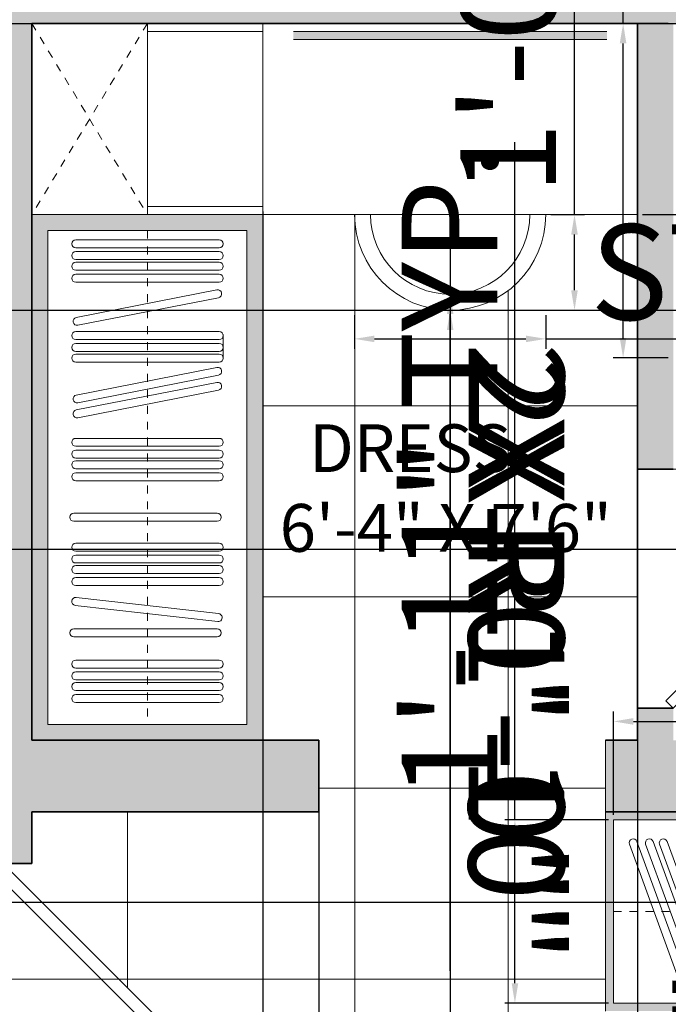
# Model space of a CAD drawing. Units: millimetres. Extents: x 542930 to 543750, y 628093 to 628738.
# Tile 9 of 14: x 543333 to 543414, y 628458 to 628581. Entities that reach past the tile are written whole.
import ezdxf

# ---------------------------------------------------------------- set-up
doc = ezdxf.new("R2010")
doc.units = ezdxf.units.MM
doc.linetypes.add('JIS_02_1.0', pattern=[2, 1, -1])
for name, color, linetype, lineweight in [('A-ANNO-DIMS', 2, 'Continuous', 18), ('A-FURN', 8, 'Continuous', 18), ('A-FURN-MILL', 8, 'Continuous', 18), ('A-FURN-MILL-HIDN', 8, 'JIS_02_1.0', 13), ('A-FURN-PATT', 9, 'Continuous', 13), ('A-WALL', 7, 'Continuous', 35), ('DOORS', 30, 'Continuous', 18)]:
    doc.layers.add(name, color=color, linetype=linetype, lineweight=lineweight)
for name, color, linetype, lineweight, true_color in [('A-AREA-IDEN', 40, 'Continuous', 18, 0xf8d731), ('A-FLOR-PATT', 241, 'Continuous', 13, 0xf7abae), ('A-WALL-PATT', 251, 'Continuous', 13, 0x636466)]:
    doc.layers.add(name, color=color, linetype=linetype, lineweight=lineweight, true_color=true_color)
doc.styles.get("Standard").update_dxf_attribs({"font": 'arial.ttf'})
doc.dimstyles.new('ISO-25', dxfattribs={"dimtxt": 12, "dimasz": 2.5, "dimexe": 1.25, "dimexo": 0.625, "dimtad": 1, "dimdec": 0, "dimlunit": 3, "dimtxsty": 'Standard', "dimcen": 2.5, "dimadec": 0, "dimazin": 0, "dimtfac": 1, "dimtdec": 0, "dimtmove": 0, "dimatfit": 3, "dimfxl": 1, "dimarcsym": 0})

# ---------------------------------------------------------------- blocks, each defined once
blk = doc.blocks.new('*U2')
for p, q in [((0, 0), (0, -6)), ((40, 0), (40, -6))]:
    blk.add_line(p, q)
blk.add_lwpolyline([(0, 0), (28.28, 28.28), (29.52, 27.05), (1.24, -1.24)], close=True)
blk.add_arc((0, 0), 40, 0, 45)
blk = doc.blocks.new('*U3')
for p, q in [((-40, 0), (-40, -6)), ((0, 0), (0, -6))]:
    blk.add_line(p, q)
blk.add_lwpolyline([(0, 0), (-28.28, 28.28), (-29.52, 27.05), (-1.24, -1.24)], close=True)
blk.add_arc((0, 0), 40, 135, 180)
blk = doc.blocks.new('WARDROBE-DRESS-RAIL')
for p, q in [((0, 0), (0, 62)), ((0, 62), (25, 62)), ((25, 0), (25, 62)), ((3.52, 60.83), (21.52, 60.83)), ((3.52, 59.83), (21.52, 59.83)), ((3.52, 59.35), (21.52, 59.35)), ((3.52, 58.35), (21.52, 58.35)), ((3.52, 58.02), (21.52, 58.02)), ((3.52, 57.02), (21.52, 57.02)), ((3.52, 56.51), (21.52, 56.51)), ((3.52, 55.51), (21.52, 55.51)), ((3.57, 51.08), (21.23, 54.55)), ((3.76, 50.1), (21.43, 53.57)), ((3.52, 49.31), (21.52, 49.31)), ((3.52, 48.31), (21.52, 48.31)), ((3.52, 47.82), (21.52, 47.82)), ((3.52, 46.82), (21.52, 46.82)), ((3.52, 46.49), (21.52, 46.49)), ((3.52, 45.49), (21.52, 45.49)), ((3.57, 41.35), (21.23, 44.82)), ((3.76, 40.37), (21.43, 43.84)), ((3.57, 39.47), (21.23, 42.94)), ((3.76, 38.49), (21.43, 41.96)), ((3.52, 35.91), (21.52, 35.91)), ((3.52, 34.91), (21.52, 34.91)), ((3.52, 34.43), (21.52, 34.43)), ((3.52, 33.43), (21.52, 33.43)), ((3.52, 33.1), (21.52, 33.1)), ((3.52, 32.1), (21.52, 32.1)), ((3.52, 31.59), (21.52, 31.59)), ((3.52, 30.59), (21.52, 30.59)), ((3.27, 26.51), (21.27, 26.51)), ((3.27, 25.51), (21.27, 25.51)), ((3.52, 22.74), (21.52, 22.74)), ((3.52, 21.74), (21.52, 21.74)), ((3.52, 21.26), (21.52, 21.26)), ((3.52, 20.26), (21.52, 20.26)), ((3.52, 19.93), (21.52, 19.93)), ((3.52, 18.93), (21.52, 18.93)), ((3.52, 18.42), (21.52, 18.42)), ((3.52, 17.42), (21.52, 17.42)), ((3.44, 14.93), (21.33, 12.92)), ((3.56, 15.93), (21.44, 13.91)), ((3.27, 11.99), (21.27, 11.99)), ((3.27, 10.99), (21.27, 10.99)), ((3.52, 8.06), (21.52, 8.06)), ((3.52, 7.06), (21.52, 7.06)), ((3.52, 6.58), (21.52, 6.58)), ((3.52, 5.58), (21.52, 5.58)), ((3.52, 5.25), (21.52, 5.25)), ((3.52, 4.25), (21.52, 4.25)), ((3.52, 3.74), (21.52, 3.74)), ((3.52, 2.74), (21.52, 2.74)), ((0, 0), (25, 0))]:
    blk.add_line(p, q)
for centre, start, end in [((3.52, 60.33), 90, 270), ((21.52, 60.33), 270, 90), ((3.52, 58.85), 90, 270), ((21.52, 58.85), 270, 90), ((3.52, 57.52), 90, 270), ((21.52, 57.52), 270, 90), ((3.52, 56.01), 90, 270), ((21.52, 56.01), 270, 90), ((21.33, 54.06), 281.1082, 101.1082), ((3.67, 50.59), 101.1082, 281.1082), ((3.52, 48.81), 90, 270), ((21.52, 48.81), 270, 90), ((3.52, 47.32), 90, 270), ((21.52, 47.32), 270, 90), ((3.52, 45.99), 90, 270), ((21.52, 45.99), 270, 90), ((21.33, 44.33), 281.1082, 101.1082), ((21.33, 42.45), 281.1082, 101.1082), ((3.67, 40.86), 101.1082, 281.1082), ((3.67, 38.98), 101.1082, 281.1082), ((3.52, 35.41), 90, 270), ((21.52, 35.41), 270, 90), ((3.52, 33.93), 90, 270), ((21.52, 33.93), 270, 90), ((3.52, 32.6), 90, 270), ((21.52, 32.6), 270, 90), ((3.52, 31.09), 90, 270), ((21.52, 31.09), 270, 90), ((3.27, 26.01), 90, 270), ((21.27, 26.01), 270, 90), ((3.52, 22.24), 90, 270), ((21.52, 22.24), 270, 90), ((3.52, 20.76), 90, 270), ((21.52, 20.76), 270, 90), ((3.52, 19.43), 90, 270), ((21.52, 19.43), 270, 90), ((3.52, 17.92), 90, 270), ((21.52, 17.92), 270, 90), ((3.5, 15.43), 83.5593, 263.5593), ((21.39, 13.41), 263.5593, 83.5611), ((3.27, 11.49), 90, 270), ((21.27, 11.49), 270, 90), ((3.52, 7.56), 90, 270), ((21.52, 7.56), 270, 90), ((3.52, 6.08), 90, 270), ((21.52, 6.08), 270, 90), ((3.52, 4.75), 90, 270), ((21.52, 4.75), 270, 90), ((3.52, 3.24), 90, 270), ((21.52, 3.24), 270, 90)]:
    blk.add_arc(centre, 0.5, start, end)
blk = doc.blocks.new('WARDROBE-BED-RAIL')
for p, q in [((0, 23), (0, 0)), ((0, 23), (82.5, 23)), ((82.5, 0), (82.5, 23)), ((14.55, 3.16), (14.55, 21.16)), ((15.55, 3.16), (15.55, 21.16)), ((34.81, 3.12), (34.81, 21.12)), ((35.81, 3.12), (35.81, 21.12)), ((36.51, 3.19), (36.51, 21.19)), ((37.51, 3.19), (37.51, 21.19)), ((38, 3.19), (38, 21.19)), ((39, 3.19), (39, 21.19)), ((8.16, 3.05), (1.98, 19.95)), ((9.1, 3.39), (2.92, 20.3)), ((10.2, 3.05), (4.02, 19.95)), ((11.14, 3.39), (4.96, 20.3)), ((11.95, 3.05), (5.77, 19.95)), ((12.89, 3.39), (6.71, 20.3)), ((17.99, 3.79), (24.17, 20.7)), ((18.92, 3.45), (25.1, 20.36)), ((19.74, 3.79), (25.92, 20.7)), ((20.68, 3.45), (26.86, 20.36)), ((21.57, 3.79), (27.75, 20.7)), ((22.51, 3.45), (28.69, 20.36)), ((31.12, 2.98), (31.12, 20.98)), ((32.12, 2.98), (32.12, 20.98)), ((33.04, 2.98), (33.04, 20.98)), ((34.04, 2.98), (34.04, 20.98)), ((41.02, 3.57), (47.2, 20.48)), ((41.96, 3.23), (48.14, 20.14)), ((42.77, 3.57), (48.95, 20.48)), ((43.71, 3.23), (49.89, 20.14)), ((44.81, 3.57), (50.99, 20.48)), ((45.75, 3.23), (51.93, 20.14)), ((53.23, 2.86), (53.23, 20.86)), ((54.23, 2.86), (54.23, 20.86)), ((55, 2.73), (55, 20.73)), ((56, 2.73), (56, 20.73)), ((56.28, 2.66), (56.28, 20.66)), ((57.28, 2.66), (57.28, 20.66)), ((57.87, 2.66), (57.87, 20.66)), ((58.87, 2.66), (58.87, 20.66)), ((59.26, 2.66), (59.26, 20.66)), ((60.26, 2.66), (60.26, 20.66)), ((60.83, 2.75), (67.01, 19.66)), ((61.77, 2.41), (67.95, 19.31)), ((62.58, 2.75), (68.76, 19.66)), ((63.52, 2.41), (69.7, 19.31)), ((68.19, 2.75), (74.37, 19.66)), ((69.13, 2.41), (75.31, 19.31)), ((69.74, 2.75), (75.92, 19.66)), ((70.68, 2.41), (76.86, 19.31)), ((0, 0), (82.5, 0))]:
    blk.add_line(p, q)
for centre, start, end in [((15.05, 21.16), 0, 180), ((24.63, 20.53), 339.919, 159.919), ((26.39, 20.53), 339.919, 159.919), ((28.22, 20.53), 339.919, 159.919), ((31.62, 20.98), 0, 180), ((33.54, 20.98), 0, 180), ((35.31, 21.12), 0, 180), ((37.01, 21.19), 0, 180), ((38.5, 21.19), 0, 180), ((53.73, 20.86), 0, 180), ((55.5, 20.73), 0, 180), ((56.78, 20.66), 0, 180), ((58.37, 20.66), 0, 180), ((59.76, 20.66), 0, 180), ((2.45, 20.12), 20.081, 200.081), ((4.49, 20.12), 20.081, 200.081), ((6.24, 20.12), 20.081, 200.081), ((47.67, 20.31), 339.919, 159.919), ((49.42, 20.31), 339.919, 159.919), ((51.46, 20.31), 339.919, 159.919), ((67.48, 19.49), 339.919, 159.919), ((69.23, 19.49), 339.919, 159.919), ((74.84, 19.49), 339.919, 159.919), ((76.39, 19.49), 339.919, 159.919), ((18.45, 3.62), 159.919, 339.919), ((20.21, 3.62), 159.919, 339.919), ((22.04, 3.62), 159.919, 339.919), ((8.63, 3.22), 200.081, 20.081), ((10.67, 3.22), 200.081, 20.081), ((12.42, 3.22), 200.081, 20.081), ((15.05, 3.16), 180, 0), ((31.62, 2.98), 180, 0), ((33.54, 2.98), 180, 0), ((35.31, 3.12), 180, 0), ((37.01, 3.19), 180, 0), ((38.5, 3.19), 180, 0), ((41.49, 3.4), 159.919, 339.919), ((43.24, 3.4), 159.919, 339.919), ((45.28, 3.4), 159.919, 339.919), ((53.73, 2.86), 180, 0), ((55.5, 2.73), 180, 0), ((56.78, 2.66), 180, 0), ((58.37, 2.66), 180, 0), ((59.76, 2.66), 180, 0), ((61.3, 2.58), 159.919, 339.919), ((63.05, 2.58), 159.919, 339.919), ((68.66, 2.58), 159.919, 339.919), ((70.21, 2.58), 159.919, 339.919)]:
    blk.add_arc(centre, 0.5, start, end)
blk = doc.blocks.new('DRESSING-STOOL')
for radius in [12, 10]:
    blk.add_arc((12, 12), radius, 180, 0)
blk = doc.blocks.new('*D37')
at = {"layer": 'A-ANNO-DIMS', "color": 0, "lineweight": -2, "transparency": 16777216}
for p, q in [((543337.17, 628423.55), (543337.17, 628436.21)), ((543417.44, 628423.55), (543417.44, 628436.21)), ((543337.17, 628434.96), (543128.93, 628434.96)), ((543414.94, 628434.96), (543339.67, 628434.96))]:
    blk.add_line(p, q, dxfattribs=at)
at = {"layer": 'A-ANNO-DIMS', "color": 0, "transparency": 16777216}
for points in [[(543339.67, 628435.38), (543339.67, 628434.55), (543337.17, 628434.96)], [(543414.94, 628435.38), (543414.94, 628434.55), (543417.44, 628434.96)]]:
    blk.add_solid(points, dxfattribs=at)
at = {"layer": 'Defpoints', "color": 0, "transparency": 16777216}
for p in [(543337.17, 628434.96), (543337.17, 628422.92), (543417.44, 628422.92)]:
    blk.add_point(p, dxfattribs=at)
at = {"layer": 'A-ANNO-DIMS', "color": 0, "transparency": 16777216, "insert": (543231.8, 628442.16), "char_height": 12, "attachment_point": 5}
blk.add_mtext('QUEEN BED 6\'-8 1/2" TYP.', dxfattribs=at)
blk = doc.blocks.new('*D38')
at = {"layer": 'A-ANNO-DIMS', "color": 0, "lineweight": -2, "transparency": 16777216}
for p, q in [((543429.48, 628422.92), (543429.48, 628499.82)), ((543418.07, 628422.92), (543430.73, 628422.92)), ((543429.48, 628365.22), (543429.48, 628420.42)), ((543418.07, 628362.72), (543430.73, 628362.72))]:
    blk.add_line(p, q, dxfattribs=at)
at = {"layer": 'A-ANNO-DIMS', "color": 0, "transparency": 16777216}
for points in [[(543429.07, 628420.42), (543429.9, 628420.42), (543429.48, 628422.92)], [(543429.07, 628365.22), (543429.9, 628365.22), (543429.48, 628362.72)]]:
    blk.add_solid(points, dxfattribs=at)
at = {"layer": 'Defpoints', "color": 0, "transparency": 16777216}
for p in [(543417.44, 628422.92), (543429.48, 628422.92), (543417.44, 628362.72)]:
    blk.add_point(p, dxfattribs=at)
at = {"layer": 'A-ANNO-DIMS', "color": 0, "transparency": 16777216, "insert": (543422.73, 628462.62), "char_height": 12, "attachment_point": 5, "rotation": 90}
blk.add_mtext('5\'-0" TYP.', dxfattribs=at)
blk = doc.blocks.new('*D45')
at = {"layer": 'A-ANNO-DIMS', "color": 0, "lineweight": -2, "transparency": 16777216}
for p, q in [((543407.17, 628481.45), (543407.17, 628494.45)), ((543489.67, 628481.45), (543489.67, 628494.45)), ((543409.67, 628493.2), (543487.17, 628493.2)), ((543489.67, 628493.2), (543749.65, 628493.2))]:
    blk.add_line(p, q, dxfattribs=at)
at = {"layer": 'A-ANNO-DIMS', "color": 0, "transparency": 16777216}
for points in [[(543409.67, 628493.62), (543409.67, 628492.78), (543407.17, 628493.2)], [(543487.17, 628493.62), (543487.17, 628492.78), (543489.67, 628493.2)]]:
    blk.add_solid(points, dxfattribs=at)
at = {"layer": 'Defpoints', "color": 0, "transparency": 16777216}
for p in [(543489.67, 628493.2), (543407.17, 628480.83), (543489.67, 628480.83)]:
    blk.add_point(p, dxfattribs=at)
at = {"layer": 'A-ANNO-DIMS', "color": 0, "transparency": 16777216, "insert": (543620.91, 628500.03), "char_height": 12, "attachment_point": 5}
blk.add_mtext('WARDROBE RAIL 6\'-10 1/2" TYP.', dxfattribs=at)
blk = doc.blocks.new('*D46')
at = {"layer": 'A-ANNO-DIMS', "color": 0, "lineweight": -2, "transparency": 16777216}
for p, q in [((543394.79, 628480.83), (543394.79, 628565.92)), ((543406.54, 628480.83), (543393.54, 628480.83)), ((543394.79, 628460.33), (543394.79, 628478.33)), ((543406.54, 628457.83), (543393.54, 628457.83))]:
    blk.add_line(p, q, dxfattribs=at)
at = {"layer": 'A-ANNO-DIMS', "color": 0, "transparency": 16777216}
for points in [[(543394.38, 628478.33), (543395.21, 628478.33), (543394.79, 628480.83)], [(543394.38, 628460.33), (543395.21, 628460.33), (543394.79, 628457.83)]]:
    blk.add_solid(points, dxfattribs=at)
at = {"layer": 'Defpoints', "color": 0, "transparency": 16777216}
for p in [(543394.79, 628480.83), (543407.17, 628480.83), (543407.17, 628457.83)]:
    blk.add_point(p, dxfattribs=at)
at = {"layer": 'A-ANNO-DIMS', "color": 0, "transparency": 16777216, "insert": (543388.14, 628524.62), "char_height": 12, "attachment_point": 5, "rotation": 90}
blk.add_mtext('1\'-11" TYP.', dxfattribs=at)
blk = doc.blocks.new('*D53')
at = {"layer": 'A-ANNO-DIMS', "color": 0, "lineweight": -2, "transparency": 16777216}
for p, q in [((543408.37, 628580.83), (543408.37, 628737.76)), ((543414.04, 628580.83), (543407.12, 628580.83)), ((543408.37, 628541.33), (543408.37, 628578.33)), ((543414.04, 628538.83), (543407.12, 628538.83))]:
    blk.add_line(p, q, dxfattribs=at)
at = {"layer": 'A-ANNO-DIMS', "color": 0, "transparency": 16777216}
for points in [[(543407.95, 628578.33), (543408.78, 628578.33), (543408.37, 628580.83)], [(543407.95, 628541.33), (543408.78, 628541.33), (543408.37, 628538.83)]]:
    blk.add_solid(points, dxfattribs=at)
at = {"layer": 'Defpoints', "color": 0, "transparency": 16777216}
for p in [(543408.37, 628580.83), (543414.67, 628580.83), (543414.67, 628538.83)]:
    blk.add_point(p, dxfattribs=at)
at = {"layer": 'A-ANNO-DIMS', "color": 0, "transparency": 16777216, "insert": (543401.53, 628660.54), "char_height": 12, "attachment_point": 5, "rotation": 90}
blk.add_mtext('SHOWER 3\'-6" TYP.', dxfattribs=at)
blk = doc.blocks.new('*D57')
at = {"layer": 'A-ANNO-DIMS', "color": 0, "lineweight": -2, "transparency": 16777216}
for p, q in [((543374.67, 628544.2), (543374.67, 628539.98)), ((543398.67, 628544.2), (543398.67, 628539.98)), ((543377.17, 628541.23), (543396.17, 628541.23)), ((543398.67, 628541.23), (543536.99, 628541.23))]:
    blk.add_line(p, q, dxfattribs=at)
at = {"layer": 'A-ANNO-DIMS', "color": 0, "transparency": 16777216}
for points in [[(543377.17, 628541.64), (543377.17, 628540.81), (543374.67, 628541.23)], [(543396.17, 628541.64), (543396.17, 628540.81), (543398.67, 628541.23)]]:
    blk.add_solid(points, dxfattribs=at)
at = {"layer": 'Defpoints', "color": 0, "transparency": 16777216}
for p in [(543374.67, 628544.83), (543398.67, 628544.83), (543398.67, 628541.23)]:
    blk.add_point(p, dxfattribs=at)
at = {"layer": 'A-ANNO-DIMS', "color": 0, "transparency": 16777216, "insert": (543469.08, 628548.06), "char_height": 12, "attachment_point": 5}
blk.add_mtext('STOOL 2\'-0" TYP.', dxfattribs=at)
blk = doc.blocks.new('*D58')
at = {"layer": 'A-ANNO-DIMS', "color": 0, "lineweight": -2, "transparency": 16777216}
for p, q in [((543402.27, 628556.83), (543402.27, 628632.59)), ((543399.29, 628556.83), (543403.52, 628556.83)), ((543402.27, 628547.33), (543402.27, 628554.33)), ((543399.29, 628544.83), (543403.52, 628544.83))]:
    blk.add_line(p, q, dxfattribs=at)
at = {"layer": 'A-ANNO-DIMS', "color": 0, "transparency": 16777216}
for points in [[(543401.85, 628554.33), (543402.68, 628554.33), (543402.27, 628556.83)], [(543401.85, 628547.33), (543402.68, 628547.33), (543402.27, 628544.83)]]:
    blk.add_solid(points, dxfattribs=at)
at = {"layer": 'Defpoints', "color": 0, "transparency": 16777216}
for p in [(543398.67, 628556.83), (543402.27, 628556.83), (543398.67, 628544.83)]:
    blk.add_point(p, dxfattribs=at)
at = {"layer": 'A-ANNO-DIMS', "color": 0, "transparency": 16777216, "insert": (543395.51, 628595.96), "char_height": 12, "attachment_point": 5, "rotation": 90}
blk.add_mtext('1\'-0" TYP.', dxfattribs=at)
blk = doc.blocks.new('*D69')
at = {"layer": 'A-ANNO-DIMS', "color": 0, "lineweight": -2, "transparency": 16777216}
for p, q in [((543271.67, 628584.95), (543271.67, 628619.78)), ((543325.17, 628581.45), (543325.17, 628619.78)), ((543274.17, 628618.53), (543322.67, 628618.53)), ((543325.17, 628618.53), (543389.26, 628618.53))]:
    blk.add_line(p, q, dxfattribs=at)
at = {"layer": 'A-ANNO-DIMS', "color": 0, "transparency": 16777216}
for points in [[(543274.17, 628618.94), (543274.17, 628618.11), (543271.67, 628618.53)], [(543322.67, 628618.94), (543322.67, 628618.11), (543325.17, 628618.53)]]:
    blk.add_solid(points, dxfattribs=at)
at = {"layer": 'Defpoints', "color": 0, "transparency": 16777216}
for p in [(543325.17, 628618.53), (543271.67, 628584.33), (543325.17, 628580.83)]:
    blk.add_point(p, dxfattribs=at)
at = {"layer": 'A-ANNO-DIMS', "color": 0, "transparency": 16777216, "insert": (543358.46, 628625.36), "char_height": 12, "attachment_point": 5}
blk.add_mtext('4\'-5 1/2"', dxfattribs=at)
blk = doc.blocks.new('*D70')
at = {"layer": 'A-ANNO-DIMS', "color": 0, "lineweight": -2, "transparency": 16777216}
for p, q in [((543325.79, 628580.83), (543537.81, 628580.83)), ((543536.56, 628517.33), (543536.56, 628578.33)), ((543325.79, 628514.83), (543537.81, 628514.83))]:
    blk.add_line(p, q, dxfattribs=at)
at = {"layer": 'A-ANNO-DIMS', "color": 0, "transparency": 16777216}
for points in [[(543536.15, 628578.33), (543536.98, 628578.33), (543536.56, 628580.83)], [(543536.15, 628517.33), (543536.98, 628517.33), (543536.56, 628514.83)]]:
    blk.add_solid(points, dxfattribs=at)
at = {"layer": 'Defpoints', "color": 0, "transparency": 16777216}
for p in [(543325.17, 628580.83), (543536.56, 628580.83), (543325.17, 628514.83)]:
    blk.add_point(p, dxfattribs=at)
at = {"layer": 'A-ANNO-DIMS', "color": 0, "transparency": 16777216, "insert": (543529.81, 628547.83), "char_height": 12, "attachment_point": 5, "rotation": 90}
blk.add_mtext('5\'-6"', dxfattribs=at)
blk = doc.blocks.new('*D72')
at = {"layer": 'A-ANNO-DIMS', "color": 0, "lineweight": -2, "transparency": 16777216}
for p, q in [((543536.56, 628544.83), (543536.56, 628580.68)), ((543282.29, 628544.83), (543537.81, 628544.83)), ((543536.56, 628517.33), (543536.56, 628542.33)), ((543282.29, 628514.83), (543537.81, 628514.83))]:
    blk.add_line(p, q, dxfattribs=at)
at = {"layer": 'A-ANNO-DIMS', "color": 0, "transparency": 16777216}
for points in [[(543536.15, 628542.33), (543536.98, 628542.33), (543536.56, 628544.83)], [(543536.15, 628517.33), (543536.98, 628517.33), (543536.56, 628514.83)]]:
    blk.add_solid(points, dxfattribs=at)
at = {"layer": 'Defpoints', "color": 0, "transparency": 16777216}
for p in [(543281.67, 628544.83), (543536.56, 628544.83), (543281.67, 628514.83)]:
    blk.add_point(p, dxfattribs=at)
at = {"layer": 'A-ANNO-DIMS', "color": 0, "transparency": 16777216, "insert": (543529.81, 628564), "char_height": 12, "attachment_point": 5, "rotation": 90}
blk.add_mtext('2\'-6"', dxfattribs=at)
blk = doc.blocks.new('*D78')
at = {"layer": 'A-ANNO-DIMS', "color": 0, "lineweight": -2, "transparency": 16777216}
for p, q in [((543304.67, 628350.45), (543304.67, 628619.78)), ((543325.17, 628350.45), (543325.17, 628619.78)), ((543307.17, 628618.53), (543322.67, 628618.53)), ((543325.17, 628618.53), (543387.65, 628618.53))]:
    blk.add_line(p, q, dxfattribs=at)
at = {"layer": 'A-ANNO-DIMS', "color": 0, "transparency": 16777216}
for points in [[(543307.17, 628618.94), (543307.17, 628618.11), (543304.67, 628618.53)], [(543322.67, 628618.94), (543322.67, 628618.11), (543325.17, 628618.53)]]:
    blk.add_solid(points, dxfattribs=at)
at = {"layer": 'Defpoints', "color": 0, "transparency": 16777216}
for p in [(543325.17, 628618.53), (543304.67, 628349.83), (543325.17, 628349.83)]:
    blk.add_point(p, dxfattribs=at)
at = {"layer": 'A-ANNO-DIMS', "color": 0, "transparency": 16777216, "insert": (543357.66, 628625.36), "char_height": 12, "attachment_point": 5}
blk.add_mtext('1\'-8 1/2"', dxfattribs=at)
blk = doc.blocks.new('*D80')
at = {"layer": 'A-ANNO-DIMS', "color": 0, "lineweight": -2, "transparency": 16777216}
for p, q in [((543228.79, 628470.52), (543537.81, 628470.52)), ((543536.56, 628437.09), (543536.56, 628468.02)), ((543228.79, 628434.59), (543537.81, 628434.59))]:
    blk.add_line(p, q, dxfattribs=at)
at = {"layer": 'A-ANNO-DIMS', "color": 0, "transparency": 16777216}
for points in [[(543536.15, 628468.02), (543536.98, 628468.02), (543536.56, 628470.52)], [(543536.15, 628437.09), (543536.98, 628437.09), (543536.56, 628434.59)]]:
    blk.add_solid(points, dxfattribs=at)
at = {"layer": 'Defpoints', "color": 0, "transparency": 16777216}
for p in [(543228.16, 628470.52), (543536.56, 628470.52), (543228.16, 628434.59)]:
    blk.add_point(p, dxfattribs=at)
at = {"layer": 'A-ANNO-DIMS', "color": 0, "transparency": 16777216, "insert": (543529.81, 628452.55), "char_height": 12, "attachment_point": 5, "rotation": 90}
blk.add_mtext('3\'-0"', dxfattribs=at)
blk = doc.blocks.new('*D82')
at = {"layer": 'A-ANNO-DIMS', "color": 0, "lineweight": -2, "transparency": 16777216}
for p, q in [((543363.17, 628557.2), (543363.17, 628103.84)), ((543410.17, 628556.2), (543410.17, 628103.84)), ((543365.67, 628105.09), (543407.67, 628105.09))]:
    blk.add_line(p, q, dxfattribs=at)
at = {"layer": 'A-ANNO-DIMS', "color": 0, "transparency": 16777216}
for points in [[(543365.67, 628105.5), (543365.67, 628104.67), (543363.17, 628105.09)], [(543407.67, 628105.5), (543407.67, 628104.67), (543410.17, 628105.09)]]:
    blk.add_solid(points, dxfattribs=at)
at = {"layer": 'Defpoints', "color": 0, "transparency": 16777216}
for p in [(543363.17, 628557.83), (543410.17, 628556.83), (543410.17, 628105.09)]:
    blk.add_point(p, dxfattribs=at)
at = {"layer": 'A-ANNO-DIMS', "color": 0, "transparency": 16777216, "insert": (543386.67, 628111.84), "char_height": 12, "attachment_point": 5}
blk.add_mtext('3\'-11"', dxfattribs=at)
blk = doc.blocks.new('*D83')
at = {"layer": 'A-ANNO-DIMS', "color": 0, "lineweight": -2, "transparency": 16777216}
for p, q in [((543536.56, 628580.83), (543536.56, 628616.68)), ((543410.79, 628580.83), (543537.81, 628580.83)), ((543536.56, 628559.33), (543536.56, 628578.33)), ((543410.79, 628556.83), (543537.81, 628556.83))]:
    blk.add_line(p, q, dxfattribs=at)
at = {"layer": 'A-ANNO-DIMS', "color": 0, "transparency": 16777216}
for points in [[(543536.15, 628578.33), (543536.98, 628578.33), (543536.56, 628580.83)], [(543536.15, 628559.33), (543536.98, 628559.33), (543536.56, 628556.83)]]:
    blk.add_solid(points, dxfattribs=at)
at = {"layer": 'Defpoints', "color": 0, "transparency": 16777216}
for p in [(543410.17, 628580.83), (543536.56, 628580.83), (543410.17, 628556.83)]:
    blk.add_point(p, dxfattribs=at)
at = {"layer": 'A-ANNO-DIMS', "color": 0, "transparency": 16777216, "insert": (543529.81, 628600), "char_height": 12, "attachment_point": 5, "rotation": 90}
blk.add_mtext('2\'-0"', dxfattribs=at)
blk = doc.blocks.new('*D84')
at = {"layer": 'A-ANNO-DIMS', "color": 0, "lineweight": -2, "transparency": 16777216}
for p, q in [((543386.67, 628556.2), (543386.67, 628103.84)), ((543370.17, 628490.2), (543370.17, 628103.84)), ((543372.67, 628105.09), (543384.17, 628105.09)), ((543386.67, 628105.09), (543449.15, 628105.09))]:
    blk.add_line(p, q, dxfattribs=at)
at = {"layer": 'A-ANNO-DIMS', "color": 0, "transparency": 16777216}
for points in [[(543372.67, 628105.5), (543372.67, 628104.67), (543370.17, 628105.09)], [(543384.17, 628105.5), (543384.17, 628104.67), (543386.67, 628105.09)]]:
    blk.add_solid(points, dxfattribs=at)
at = {"layer": 'Defpoints', "color": 0, "transparency": 16777216}
for p in [(543386.67, 628556.83), (543370.17, 628490.83), (543386.67, 628105.09)]:
    blk.add_point(p, dxfattribs=at)
at = {"layer": 'A-ANNO-DIMS', "color": 0, "transparency": 16777216, "insert": (543419.16, 628111.92), "char_height": 12, "attachment_point": 5}
blk.add_mtext('1\'-4 1/2"', dxfattribs=at)
blk = doc.blocks.new('*D90')
at = {"layer": 'A-ANNO-DIMS', "color": 0, "lineweight": -2, "transparency": 16777216}
for p, q in [((543386.67, 628556.83), (543386.67, 628546.83)), ((543386.67, 628461.88), (543386.67, 628544.33))]:
    blk.add_line(p, q, dxfattribs=at)
at = {"layer": 'A-ANNO-DIMS', "color": 0, "transparency": 16777216}
blk.add_solid([(543387.08, 628544.33), (543386.25, 628544.33), (543386.67, 628546.83)], dxfattribs=at)
at = {"layer": 'Defpoints', "color": 0, "transparency": 16777216}
for p in [(543386.67, 628556.83), (543386.67, 628546.83)]:
    blk.add_point(p, dxfattribs=at)
at = {"layer": 'A-ANNO-DIMS', "color": 0, "transparency": 16777216, "insert": (543393.42, 628501.85), "char_height": 12, "attachment_point": 5, "rotation": 270.0007}
blk.add_mtext('2X R0\'-10"', dxfattribs=at)
blk = doc.blocks.new('*D91')
at = {"layer": 'A-ANNO-DIMS', "color": 0, "lineweight": -2, "transparency": 16777216}
for p, q in [((543386.67, 628556.83), (543386.67, 628544.83)), ((543386.67, 628469.2), (543386.67, 628542.33))]:
    blk.add_line(p, q, dxfattribs=at)
at = {"layer": 'A-ANNO-DIMS', "color": 0, "transparency": 16777216}
blk.add_solid([(543387.08, 628542.33), (543386.25, 628542.33), (543386.67, 628544.83)], dxfattribs=at)
at = {"layer": 'Defpoints', "color": 0, "transparency": 16777216}
for p in [(543386.67, 628556.83), (543386.67, 628544.83)]:
    blk.add_point(p, dxfattribs=at)
at = {"layer": 'A-ANNO-DIMS', "color": 0, "transparency": 16777216, "insert": (543393.42, 628504.51), "char_height": 12, "attachment_point": 5, "rotation": 270.0006}
blk.add_mtext('2X R1\'-0"', dxfattribs=at)

msp = doc.modelspace()

# ---------------------------------------------------------------- hatches: boundary and pattern name
at = {"layer": 'A-FURN-PATT'}
h = msp.add_hatch(color=256, dxfattribs=at)
h.dxf.hatch_style = 1
h.paths.add_polyline_path([(543406.34, 628579.83), (543366.99, 628579.83), (543366.99, 628578.83), (543406.34, 628578.83)])
h = msp.add_hatch(color=256, dxfattribs=at)
h.dxf.hatch_style = 1
h.paths.add_polyline_path([(543363.17, 628556.83), (543334.17, 628556.83), (543334.17, 628490.83), (543363.17, 628490.83)])
h.paths.add_polyline_path([(543361.17, 628492.83), (543336.17, 628492.83), (543336.17, 628554.83), (543361.17, 628554.83)], flags=16)
h.paths.add_polyline_path([(543357.69, 628552.66), (543348.67, 628552.66), (543348.67, 628552.17), (543357.69, 628552.17, -1), (543357.69, 628551.17), (543348.67, 628551.17), (543348.67, 628550.84), (543357.69, 628550.84, -1), (543357.69, 628549.84), (543348.67, 628549.84), (543348.67, 628549.33), (543357.69, 628549.33, -1), (543357.69, 628548.33), (543348.67, 628548.33), (543348.67, 628545.66), (543357.4, 628547.38, -1.000014), (543357.59, 628546.4), (543348.67, 628544.64), (543348.67, 628542.13), (543357.69, 628542.13, -0.50839), (543358.17, 628541.48), (543358.17, 628540.3, -0.156536), (543358.17, 628539.99), (543358.17, 628538.97, -0.50839), (543357.69, 628538.32), (543348.67, 628538.32), (543348.67, 628535.93), (543357.4, 628537.65, -1.000014), (543357.59, 628536.67), (543348.67, 628534.91), (543348.67, 628534.05), (543357.4, 628535.76, -1.000014), (543357.59, 628534.78), (543348.67, 628533.03), (543348.67, 628528.74), (543357.69, 628528.74, -1), (543357.69, 628527.74), (543348.67, 628527.74), (543348.67, 628527.25), (543357.69, 628527.25, -1), (543357.69, 628526.25), (543348.67, 628526.25), (543348.67, 628525.93), (543357.69, 628525.93, -1), (543357.69, 628524.93), (543348.67, 628524.93), (543348.67, 628524.41), (543357.69, 628524.41, -1), (543357.69, 628523.41), (543348.67, 628523.41), (543348.67, 628519.34), (543357.44, 628519.34, -1), (543357.44, 628518.34), (543348.67, 628518.34), (543348.67, 628515.57), (543357.69, 628515.57, -1), (543357.69, 628514.57), (543348.67, 628514.57), (543348.67, 628514.08), (543357.69, 628514.08, -1), (543357.69, 628513.08), (543348.67, 628513.08), (543348.67, 628512.76), (543357.69, 628512.76, -1), (543357.69, 628511.76), (543348.67, 628511.76), (543348.67, 628511.24), (543357.69, 628511.24, -1), (543357.69, 628510.24), (543348.67, 628510.24), (543348.67, 628507.74), (543357.61, 628506.73, -1.000011), (543357.5, 628505.74), (543348.67, 628506.74), (543348.67, 628504.81), (543357.44, 628504.81, -1), (543357.44, 628503.81), (543348.67, 628503.81), (543348.67, 628500.89), (543357.69, 628500.89, -1), (543357.69, 628499.89), (543348.67, 628499.89), (543348.67, 628499.4), (543357.69, 628499.4, -1), (543357.69, 628498.4), (543348.67, 628498.4), (543348.67, 628498.08), (543357.69, 628498.08, -1), (543357.69, 628497.08), (543348.67, 628497.08), (543348.67, 628496.56), (543357.69, 628496.56, -1), (543357.69, 628495.56), (543339.69, 628495.56, -1), (543339.69, 628496.56), (543348.67, 628496.56), (543348.67, 628497.08), (543339.69, 628497.08, -1), (543339.69, 628498.08), (543348.67, 628498.08), (543348.67, 628498.4), (543339.69, 628498.4, -1), (543339.69, 628499.4), (543348.67, 628499.4), (543348.67, 628499.89), (543339.69, 628499.89, -1), (543339.69, 628500.89), (543348.67, 628500.89), (543348.67, 628503.81), (543339.44, 628503.81, -1), (543339.44, 628504.81), (543348.67, 628504.81), (543348.67, 628506.74), (543339.61, 628507.76, -0.999984), (543339.72, 628508.75), (543348.67, 628507.74), (543348.67, 628510.24), (543339.69, 628510.24, -1), (543339.69, 628511.24), (543348.67, 628511.24), (543348.67, 628511.76), (543339.69, 628511.76, -1), (543339.69, 628512.76), (543348.67, 628512.76), (543348.67, 628513.08), (543339.69, 628513.08, -1), (543339.69, 628514.08), (543348.67, 628514.08), (543348.67, 628514.57), (543339.69, 628514.57, -1), (543339.69, 628515.57), (543348.67, 628515.57), (543348.67, 628518.34), (543339.44, 628518.34, -1), (543339.44, 628519.34), (543348.67, 628519.34), (543348.67, 628523.41), (543339.69, 628523.41, -1), (543339.69, 628524.41), (543348.67, 628524.41), (543348.67, 628524.93), (543339.69, 628524.93, -1), (543339.69, 628525.93), (543348.67, 628525.93), (543348.67, 628526.25), (543339.69, 628526.25, -1), (543339.69, 628527.25), (543348.67, 628527.25), (543348.67, 628527.74), (543339.69, 628527.74, -1), (543339.69, 628528.74), (543348.67, 628528.74), (543348.67, 628533.03), (543339.93, 628531.31, -1.000015), (543339.74, 628532.29), (543348.67, 628534.05), (543348.67, 628534.91), (543339.93, 628533.2, -1.000015), (543339.74, 628534.18), (543348.67, 628535.93), (543348.67, 628538.32), (543339.69, 628538.32, -1), (543339.69, 628539.32), (543348.67, 628539.32), (543348.67, 628539.65), (543339.69, 628539.65, -1), (543339.69, 628540.65), (543348.67, 628540.65), (543348.67, 628541.13), (543339.69, 628541.13, -1), (543339.69, 628542.13), (543348.67, 628542.13), (543348.67, 628544.64), (543339.93, 628542.93, -1.000015), (543339.74, 628543.91), (543348.67, 628545.66), (543348.67, 628548.33), (543339.69, 628548.33, -1), (543339.69, 628549.33), (543348.67, 628549.33), (543348.67, 628549.84), (543339.69, 628549.84, -1), (543339.69, 628550.84), (543348.67, 628550.84), (543348.67, 628551.17), (543339.69, 628551.17, -1), (543339.69, 628552.17), (543348.67, 628552.17), (543348.67, 628552.66), (543339.69, 628552.66, -1), (543339.69, 628553.66), (543357.69, 628553.66, -1)], flags=0)
h = msp.add_hatch(color=256, dxfattribs=at)
h.dxf.hatch_style = 1
h.paths.add_polyline_path([(543490.67, 628481.83), (543406.17, 628481.83), (543406.17, 628456.83), (543490.67, 628456.83)])
h.paths.add_polyline_path([(543407.17, 628480.83), (543489.67, 628480.83), (543489.67, 628457.83), (543407.17, 628457.83)], flags=16)
h.paths.add_polyline_path([(543409.15, 628477.78, -1), (543410.09, 628478.12), (543413.3, 628469.33), (543414.27, 628469.33), (543411.18, 628477.78, -1), (543412.12, 628478.12), (543415.34, 628469.33), (543416.03, 628469.33), (543412.94, 628477.78, -1), (543413.88, 628478.12), (543417.09, 628469.33), (543421.72, 628469.33), (543421.72, 628478.99, -1), (543422.72, 628478.99), (543422.72, 628469.33), (543427.97, 628469.33), (543431.33, 628478.53, -1), (543432.27, 628478.18), (543429.03, 628469.33), (543429.72, 628469.33), (543433.09, 628478.53, -1), (543434.03, 628478.18), (543430.79, 628469.33), (543431.55, 628469.33), (543434.91, 628478.53, -1), (543435.85, 628478.18), (543432.61, 628469.33), (543438.29, 628469.33), (543438.29, 628478.81, -1), (543439.29, 628478.81), (543439.29, 628469.33), (543440.2, 628469.33), (543440.2, 628478.81, -1), (543441.2, 628478.81), (543441.2, 628469.33), (543441.98, 628469.33), (543441.98, 628478.95, -1), (543442.98, 628478.95), (543442.98, 628469.33), (543443.68, 628469.33), (543443.68, 628479.02, -1), (543444.68, 628479.02), (543444.68, 628469.33), (543445.17, 628469.33), (543445.17, 628479.02, -1), (543446.17, 628479.02), (543446.17, 628469.33), (543451.08, 628469.33), (543454.37, 628478.31, -1), (543455.31, 628477.96), (543452.15, 628469.33), (543452.84, 628469.33), (543456.12, 628478.31, -1), (543457.06, 628477.96), (543453.9, 628469.33), (543454.88, 628469.33), (543458.16, 628478.31, -1), (543459.1, 628477.96), (543455.94, 628469.33), (543460.39, 628469.33), (543460.39, 628478.68, -1), (543461.39, 628478.68), (543461.39, 628469.33), (543462.17, 628469.33), (543462.17, 628478.56, -1), (543463.17, 628478.56), (543463.17, 628469.33), (543463.45, 628469.33), (543463.45, 628478.49, -1), (543464.45, 628478.49), (543464.45, 628469.33), (543465.03, 628469.33), (543465.03, 628478.49, -1), (543466.03, 628478.49), (543466.03, 628469.33), (543466.43, 628469.33), (543466.43, 628478.49, -1), (543467.43, 628478.49), (543467.43, 628469.33), (543471.19, 628469.33), (543474.18, 628477.48, -1), (543475.11, 628477.14), (543472.26, 628469.33), (543472.95, 628469.33), (543475.93, 628477.48, -1), (543476.87, 628477.14), (543474.01, 628469.33), (543478.55, 628469.33), (543481.53, 628477.48, -1), (543482.47, 628477.14), (543479.62, 628469.33), (543480.1, 628469.33), (543483.09, 628477.48, -1), (543484.02, 628477.14), (543477.84, 628460.23, -1), (543476.91, 628460.58), (543480.1, 628469.33), (543479.62, 628469.33), (543476.29, 628460.23, -1), (543475.35, 628460.58), (543478.55, 628469.33), (543474.01, 628469.33), (543470.69, 628460.23, -1), (543469.75, 628460.58), (543472.95, 628469.33), (543472.26, 628469.33), (543468.93, 628460.23, -1), (543468, 628460.58), (543471.19, 628469.33), (543467.43, 628469.33), (543467.43, 628460.49, -1), (543466.43, 628460.49), (543466.43, 628469.33), (543466.03, 628469.33), (543466.03, 628460.49, -1), (543465.03, 628460.49), (543465.03, 628469.33), (543464.45, 628469.33), (543464.45, 628460.49, -1), (543463.45, 628460.49), (543463.45, 628469.33), (543463.17, 628469.33), (543463.17, 628460.56, -1), (543462.17, 628460.56), (543462.17, 628469.33), (543461.39, 628469.33), (543461.39, 628460.68, -1), (543460.39, 628460.68), (543460.39, 628469.33), (543455.94, 628469.33), (543452.92, 628461.06, -1), (543451.98, 628461.4), (543454.88, 628469.33), (543453.9, 628469.33), (543450.88, 628461.06, -1), (543449.94, 628461.4), (543452.84, 628469.33), (543452.15, 628469.33), (543449.13, 628461.06, -1), (543448.19, 628461.4), (543451.08, 628469.33), (543446.17, 628469.33), (543446.17, 628461.02, -1), (543445.17, 628461.02), (543445.17, 628469.33), (543444.68, 628469.33), (543444.68, 628461.02, -1), (543443.68, 628461.02), (543443.68, 628469.33), (543442.98, 628469.33), (543442.98, 628460.95, -1), (543441.98, 628460.95), (543441.98, 628469.33), (543441.2, 628469.33), (543441.2, 628460.81, -1), (543440.2, 628460.81), (543440.2, 628469.33), (543439.29, 628469.33), (543439.29, 628460.81, -1), (543438.29, 628460.81), (543438.29, 628469.33), (543432.61, 628469.33), (543429.67, 628461.28, -1), (543428.73, 628461.62), (543431.55, 628469.33), (543430.79, 628469.33), (543427.85, 628461.28, -1), (543426.91, 628461.62), (543429.72, 628469.33), (543429.03, 628469.33), (543426.09, 628461.28, -1), (543425.15, 628461.62), (543427.97, 628469.33), (543422.72, 628469.33), (543422.72, 628460.99, -1), (543421.72, 628460.99), (543421.72, 628469.33), (543417.09, 628469.33), (543420.06, 628461.22, -1), (543419.12, 628460.87), (543416.03, 628469.33), (543415.34, 628469.33), (543418.3, 628461.22, -1), (543417.36, 628460.87), (543414.27, 628469.33), (543413.3, 628469.33), (543416.27, 628461.22, -1), (543415.33, 628460.87)], flags=0)
at = {"layer": 'A-WALL-PATT'}
h = msp.add_hatch(color=256, dxfattribs=at)
h.dxf.hatch_style = 1
h.paths.add_polyline_path([(543454.53, 628589.83), (543271.67, 628589.83), (543271.67, 628580.83), (543325.17, 628580.83), (543325.17, 628475.36), (543334.17, 628475.36), (543334.17, 628481.83), (543370.17, 628481.83), (543370.17, 628490.83), (543334.17, 628490.83), (543334.17, 628580.83), (543410.17, 628580.83), (543410.17, 628524.86), (543414.67, 628524.86), (543414.67, 628580.83), (543454.53, 628580.83)])
h = msp.add_hatch(color=256, dxfattribs=at)
h.dxf.hatch_style = 1
h.paths.add_polyline_path([(543499.67, 628589.83), (543478.53, 628589.83), (543478.53, 628580.83), (543490.67, 628580.83), (543490.67, 628490.83), (543414.67, 628490.83), (543414.67, 628494.86), (543410.17, 628494.86), (543410.17, 628490.83), (543406.17, 628490.83), (543406.17, 628481.83), (543490.67, 628481.83), (543490.67, 628340.3), (543499.67, 628340.3)])

# ---------------------------------------------------------------- linework, layer by layer
at = {"layer": 'A-FLOR-PATT'}
for p, q in [((543374.7, 628423.51), (543374.7, 628556.83)), ((543393.93, 628423.51), (543393.93, 628547.28)), ((543358.17, 628538.67), (543358.17, 628541.79)), ((543363.17, 628532.83), (543410.17, 628532.83)), ((543363.17, 628508.83), (543410.17, 628508.83)), ((543370.17, 628484.83), (543406.17, 628484.83)), ((543346.17, 628459.76), (543346.17, 628481.83)), ((543228.16, 628460.83), (543406.17, 628460.83))]:
    msp.add_line(p, q, dxfattribs=at)
at = {"layer": 'A-FURN-MILL'}
for p, q in [((543348.67, 628556.83), (543348.67, 628580.83)), ((543363.17, 628490.83), (543363.17, 628580.83)), ((543348.67, 628579.83), (543363.17, 628579.83)), ((543366.99, 628579.83), (543406.34, 628579.83)), ((543366.99, 628578.83), (543406.34, 628578.83)), ((543334.17, 628556.83), (543410.17, 628556.83)), ((543348.67, 628557.83), (543363.17, 628557.83)), ((543406.17, 628490.83), (543406.17, 628456.83))]:
    msp.add_line(p, q, dxfattribs=at)
at = {"layer": 'A-FURN-MILL-HIDN'}
for p, q in [((543334.17, 628580.83), (543348.67, 628556.83)), ((543348.67, 628580.83), (543334.17, 628556.83)), ((543348.67, 628554.83), (543348.67, 628492.83)), ((543407.17, 628469.33), (543489.67, 628469.33))]:
    msp.add_line(p, q, dxfattribs=at)
at = {"layer": 'A-WALL'}
for p, q in [((543334.17, 628490.83), (543334.17, 628580.83)), ((543334.17, 628580.83), (543410.17, 628580.83)), ((543410.17, 628490.83), (543410.17, 628580.83)), ((543410.17, 628524.86), (543414.67, 628524.86)), ((543410.17, 628494.86), (543414.67, 628494.86)), ((543370.17, 628490.83), (543334.17, 628490.83)), ((543370.17, 628481.83), (543370.17, 628490.83)), ((543410.17, 628490.83), (543406.17, 628490.83)), ((543370.17, 628481.83), (543334.17, 628481.83)), ((543334.17, 628475.36), (543334.17, 628481.83)), ((543490.67, 628481.83), (543406.17, 628481.83)), ((543334.17, 628475.36), (543325.17, 628475.36))]:
    msp.add_line(p, q, dxfattribs=at)

# ---------------------------------------------------------------- block references
at = {"layer": 'A-FURN'}
msp.add_blockref('DRESSING-STOOL', (543374.67, 628544.83), dxfattribs=at)
at = {"layer": 'A-FURN-MILL'}
for name, p in [('WARDROBE-DRESS-RAIL', (543336.17, 628492.83)), ('WARDROBE-BED-RAIL', (543407.17, 628457.83))]:
    msp.add_blockref(name, p, dxfattribs=at)
at = {"layer": 'DOORS', "rotation": 270}
for name, p, xscale, yscale, zscale in [('*U3', (543414.67, 628494.86), 0.75, 0.75, 0.75), ('*U2', (543330.57, 628475.36), 0.8999999999970896, 0.8999999999970896, 0.8999999999970896)]:
    msp.add_blockref(name, p, dxfattribs=dict(at, xscale=xscale, yscale=yscale, zscale=zscale))

# ---------------------------------------------------------------- texts
at = {"layer": 'A-AREA-IDEN', "insert": (543365.28, 628530.5), "char_height": 6, "attachment_point": 1}
msp.add_mtext_dynamic_manual_height_columns('  DRESS\\P6\'-4" X 7\'6"', width=44.748, gutter_width=12.5, heights=[0], dxfattribs=at)

# ---------------------------------------------------------------- dimensions: what is measured, and where the dimension line sits
at = {"layer": 'A-ANNO-DIMS'}
for base, p1, p2, angle, text, picture, middle in [((543408.37, 628580.83), (543414.67, 628538.83), (543414.67, 628580.83), 90, 'SHOWER <> TYP.', '*D53', (543401.53, 628660.54)), ((543402.27, 628556.83), (543398.67, 628544.83), (543398.67, 628556.83), 90, '<> TYP.', '*D58', (543395.51, 628595.96)), ((543394.79, 628480.83), (543407.17, 628457.83), (543407.17, 628480.83), 90, '<> TYP.', '*D46', (543388.14, 628524.62)), ((543429.48, 628422.92), (543417.44, 628362.72), (543417.44, 628422.92), 90, '<> TYP.', '*D38', (543422.73, 628462.62)), ((543337.17, 628434.96), (543417.44, 628422.92), (543337.17, 628422.92), 180, 'QUEEN BED <> TYP.', '*D37', (543231.8, 628442.16))]:
    dim = msp.add_linear_dim(base=base, p1=p1, p2=p2, angle=angle, text=text, dimstyle='ISO-25', override={"dimdec": 1, "dimlfac": 1, "dimrnd": 0, "dimzin": 1, "dimdsep": 46, "dimlunit": 4, "dimfrac": 2}, dxfattribs=at)
    dim.commit()
    dim.dimension.update_dxf_attribs({"geometry": picture, "text_midpoint": middle})
for base, p1, p2, picture, middle in [((543325.17, 628618.53), (543271.67, 628584.33), (543325.17, 628580.83), '*D69', (543358.46, 628625.36)), ((543325.17, 628618.53), (543304.67, 628349.83), (543325.17, 628349.83), '*D78', (543357.66, 628625.36)), ((543410.17, 628105.09), (543363.17, 628557.83), (543410.17, 628556.83), '*D82', (543386.67, 628111.84)), ((543386.67, 628105.09), (543370.17, 628490.83), (543386.67, 628556.83), '*D84', (543419.16, 628111.92))]:
    dim = msp.add_linear_dim(base=base, p1=p1, p2=p2, dimstyle='ISO-25', override={"dimdec": 1, "dimlfac": 1, "dimrnd": 0, "dimzin": 1, "dimdsep": 46, "dimlunit": 4, "dimfrac": 2}, dxfattribs=at)
    dim.commit()
    dim.dimension.update_dxf_attribs({"geometry": picture, "text_midpoint": middle})
for base, p1, p2, picture, middle in [((543536.56, 628580.83), (543410.17, 628556.83), (543410.17, 628580.83), '*D83', (543529.81, 628600)), ((543536.56, 628544.83), (543281.67, 628514.83), (543281.67, 628544.83), '*D72', (543529.81, 628564)), ((543536.56, 628580.83), (543325.17, 628514.83), (543325.17, 628580.83), '*D70', (543529.81, 628547.83)), ((543536.56, 628470.52), (543228.16, 628434.59), (543228.16, 628470.52), '*D80', (543529.81, 628452.55))]:
    dim = msp.add_linear_dim(base=base, p1=p1, p2=p2, angle=90, dimstyle='ISO-25', override={"dimdec": 1, "dimlfac": 1, "dimrnd": 0, "dimzin": 1, "dimdsep": 46, "dimlunit": 4, "dimfrac": 2}, dxfattribs=at)
    dim.commit()
    dim.dimension.update_dxf_attribs({"geometry": picture, "text_midpoint": middle})
for base, p1, p2, text, picture, middle in [((543398.67, 628541.23), (543374.67, 628544.83), (543398.67, 628544.83), 'STOOL <> TYP.', '*D57', (543469.08, 628548.06)), ((543489.67, 628493.2), (543407.17, 628480.83), (543489.67, 628480.83), 'WARDROBE RAIL <> TYP.', '*D45', (543620.91, 628500.03))]:
    dim = msp.add_linear_dim(base=base, p1=p1, p2=p2, text=text, dimstyle='ISO-25', override={"dimdec": 1, "dimlfac": 1, "dimrnd": 0, "dimzin": 1, "dimdsep": 46, "dimlunit": 4, "dimfrac": 2}, dxfattribs=at)
    dim.commit()
    dim.dimension.update_dxf_attribs({"geometry": picture, "text_midpoint": middle})
for mpoint, picture, middle in [((543386.67, 628546.83), '*D90', (543393.42, 628501.85)), ((543386.67, 628544.83), '*D91', (543393.42, 628504.51))]:
    dim = msp.add_radius_dim(center=(543386.67, 628556.83), mpoint=mpoint, text='2X <>', dimstyle='ISO-25', override={"dimdec": 1, "dimlfac": 1, "dimrnd": 0, "dimzin": 1, "dimdsep": 46, "dimlunit": 4, "dimfrac": 2}, dxfattribs=at)
    dim.commit()
    dim.dimension.update_dxf_attribs({"geometry": picture, "text_midpoint": middle})

doc.saveas('drawing.dxf')
